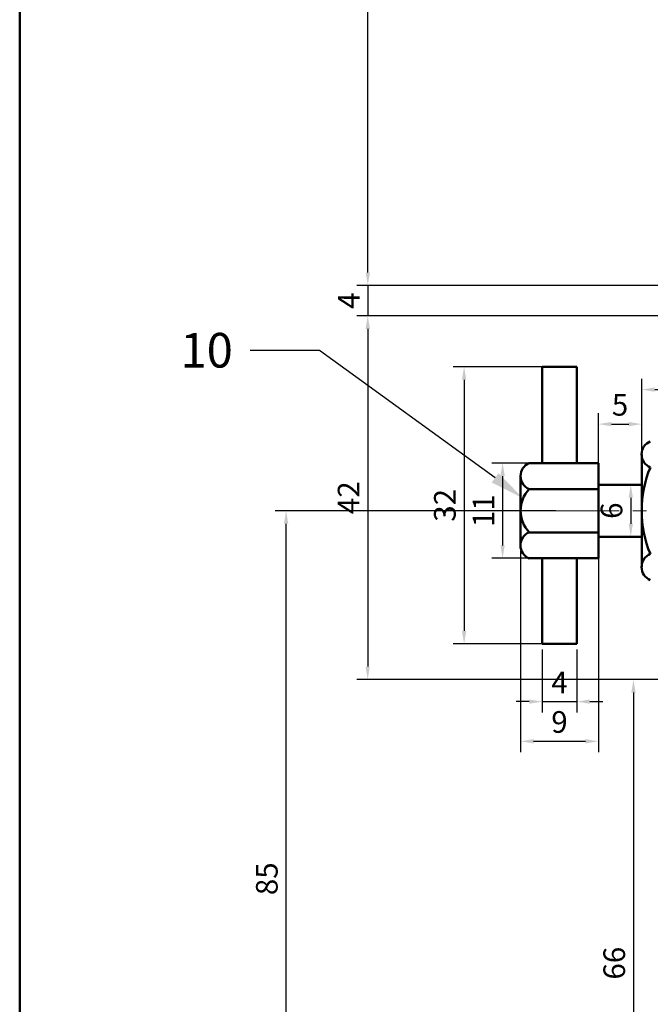
# Model space of a CAD drawing. Units: millimetres. Extents: x -414 to 17, y 81 to 417.
# Tile 2 of 7: x -414 to -341, y 143 to 257. Entities that reach past the tile are written whole.
import ezdxf
from ezdxf import colors
from ezdxf.entities.mleader import LeaderData, LeaderLine
from ezdxf.math import Vec2, Vec3

# ---------------------------------------------------------------- set-up
doc = ezdxf.new("R2010")
doc.units = ezdxf.units.MM
doc.header["$LTSCALE"] = 0.5
doc.linetypes.add('CENTER', pattern=[50.8, 31.75, -6.35, 6.35, -6.35])
for name, color, linetype, lineweight in [('M-CNTR', 1, 'CENTER', 18), ('M-DIMS', 2, 'Continuous', 25), ('M-OUTL', 7, 'Continuous', 50)]:
    doc.layers.add(name, color=color, linetype=linetype, lineweight=lineweight)
doc.styles.get("Standard").update_dxf_attribs({"font": 'arial.ttf'})
doc.dimstyles.new('ISO-25', dxfattribs={"dimtxt": 2.5, "dimasz": 1.5, "dimexe": 1.25, "dimexo": 0.625, "dimtad": 1, "dimtoh": 1, "dimdec": 0, "dimtxsty": 'Standard', "dimcen": 2.5, "dimadec": 0, "dimazin": 0, "dimtfac": 1, "dimtdec": 0, "dimtmove": 0, "dimatfit": 3, "dimfxl": 1, "dimarcsym": 0})

# ---------------------------------------------------------------- blocks, each defined once
blk = doc.blocks.new('*D30')
at = {"layer": 'Defpoints', "color": 0, "ltscale": 0.5, "transparency": 16777216}
for p in [(-330.49, 214.44), (-330.49, 209.27), (-342.49, 205.1)]:
    blk.add_point(p, dxfattribs=at)
at = {"layer": 'M-DIMS', "color": 0, "lineweight": -2, "ltscale": 0.5, "transparency": 16777216}
for p, q in [((-342.49, 205.73), (-342.49, 215.69)), ((-330.49, 209.89), (-330.49, 215.69)), ((-340.99, 214.44), (-331.99, 214.44))]:
    blk.add_line(p, q, dxfattribs=at)
at = {"layer": 'M-DIMS', "color": 0, "ltscale": 0.5, "transparency": 16777216}
for points in [[(-340.99, 214.69), (-340.99, 214.19), (-342.49, 214.44)], [(-331.99, 214.69), (-331.99, 214.19), (-330.49, 214.44)]]:
    blk.add_solid(points, dxfattribs=at)
at = {"layer": 'M-DIMS', "color": 0, "ltscale": 0.5, "transparency": 16777216, "insert": (-336.49, 216.32), "char_height": 2.5, "attachment_point": 5}
blk.add_mtext('12', dxfattribs=at)
blk = doc.blocks.new('*D32')
at = {"layer": 'Defpoints', "color": 0, "ltscale": 0.5, "transparency": 16777216}
for p in [(-344.99, 203.46), (-344.99, 197.46), (-343.75, 197.46)]:
    blk.add_point(p, dxfattribs=at)
at = {"layer": 'M-DIMS', "color": 0, "lineweight": -2, "ltscale": 0.5, "transparency": 16777216}
for p, q in [((-344.37, 203.46), (-342.5, 203.46)), ((-343.75, 201.96), (-343.75, 198.96)), ((-344.37, 197.46), (-342.5, 197.46))]:
    blk.add_line(p, q, dxfattribs=at)
at = {"layer": 'M-DIMS', "color": 0, "ltscale": 0.5, "transparency": 16777216}
for points in [[(-344, 201.96), (-343.5, 201.96), (-343.75, 203.46)], [(-344, 198.96), (-343.5, 198.96), (-343.75, 197.46)]]:
    blk.add_solid(points, dxfattribs=at)
at = {"layer": 'M-DIMS', "color": 0, "ltscale": 0.5, "transparency": 16777216, "insert": (-345.65, 200.46), "char_height": 2.5, "attachment_point": 5, "rotation": 90}
blk.add_mtext('6', dxfattribs=at)
blk = doc.blocks.new('*D33')
at = {"layer": 'Defpoints', "color": 0, "ltscale": 0.5, "transparency": 16777216}
for p in [(-342.49, 210.46), (-347.49, 203.46), (-342.49, 203.46)]:
    blk.add_point(p, dxfattribs=at)
at = {"layer": 'M-DIMS', "color": 0, "lineweight": -2, "ltscale": 0.5, "transparency": 16777216}
for p, q in [((-347.49, 204.09), (-347.49, 211.71)), ((-342.49, 204.09), (-342.49, 211.71)), ((-345.99, 210.46), (-343.99, 210.46))]:
    blk.add_line(p, q, dxfattribs=at)
at = {"layer": 'M-DIMS', "color": 0, "ltscale": 0.5, "transparency": 16777216}
for points in [[(-345.99, 210.71), (-345.99, 210.21), (-347.49, 210.46)], [(-343.99, 210.71), (-343.99, 210.21), (-342.49, 210.46)]]:
    blk.add_solid(points, dxfattribs=at)
at = {"layer": 'M-DIMS', "color": 0, "ltscale": 0.5, "transparency": 16777216, "insert": (-344.99, 212.36), "char_height": 2.5, "attachment_point": 5}
blk.add_mtext('5', dxfattribs=at)
blk = doc.blocks.new('*D34')
at = {"layer": 'Defpoints', "color": 0, "ltscale": 0.5, "transparency": 16777216}
for p in [(-353.99, 185.08), (-349.99, 185.08), (-349.99, 178.41)]:
    blk.add_point(p, dxfattribs=at)
at = {"layer": 'M-DIMS', "color": 0, "lineweight": -2, "ltscale": 0.5, "transparency": 16777216}
for p, q in [((-353.99, 184.45), (-353.99, 177.16)), ((-349.99, 184.45), (-349.99, 177.16)), ((-355.49, 178.41), (-356.99, 178.41)), ((-353.99, 178.41), (-349.99, 178.41)), ((-348.49, 178.41), (-346.99, 178.41))]:
    blk.add_line(p, q, dxfattribs=at)
at = {"layer": 'M-DIMS', "color": 0, "ltscale": 0.5, "transparency": 16777216}
for points in [[(-355.49, 178.66), (-355.49, 178.16), (-353.99, 178.41)], [(-348.49, 178.66), (-348.49, 178.16), (-349.99, 178.41)]]:
    blk.add_solid(points, dxfattribs=at)
at = {"layer": 'M-DIMS', "color": 0, "ltscale": 0.5, "transparency": 16777216, "insert": (-351.99, 180.29), "char_height": 2.5, "attachment_point": 5}
blk.add_mtext('4', dxfattribs=at)
blk = doc.blocks.new('*D35')
at = {"layer": 'Defpoints', "color": 0, "ltscale": 0.5, "transparency": 16777216}
for p in [(-356.49, 196.46), (-347.49, 196.46), (-347.49, 173.83)]:
    blk.add_point(p, dxfattribs=at)
at = {"layer": 'M-DIMS', "color": 0, "lineweight": -2, "ltscale": 0.5, "transparency": 16777216}
for p, q in [((-356.49, 195.84), (-356.49, 172.58)), ((-347.49, 195.84), (-347.49, 172.58)), ((-354.99, 173.83), (-348.99, 173.83))]:
    blk.add_line(p, q, dxfattribs=at)
at = {"layer": 'M-DIMS', "color": 0, "ltscale": 0.5, "transparency": 16777216}
for points in [[(-354.99, 174.08), (-354.99, 173.58), (-356.49, 173.83)], [(-348.99, 174.08), (-348.99, 173.58), (-347.49, 173.83)]]:
    blk.add_solid(points, dxfattribs=at)
at = {"layer": 'M-DIMS', "color": 0, "ltscale": 0.5, "transparency": 16777216, "insert": (-351.99, 175.74), "char_height": 2.5, "attachment_point": 5}
blk.add_mtext('9', dxfattribs=at)
blk = doc.blocks.new('*D36')
at = {"layer": 'Defpoints', "color": 0, "ltscale": 0.5, "transparency": 16777216}
for p in [(-351.99, 217.08), (-363.01, 185.08), (-351.99, 185.08)]:
    blk.add_point(p, dxfattribs=at)
at = {"layer": 'M-DIMS', "color": 0, "lineweight": -2, "ltscale": 0.5, "transparency": 16777216}
for p, q in [((-352.62, 217.08), (-364.26, 217.08)), ((-363.01, 215.58), (-363.01, 186.58)), ((-352.62, 185.08), (-364.26, 185.08))]:
    blk.add_line(p, q, dxfattribs=at)
at = {"layer": 'M-DIMS', "color": 0, "ltscale": 0.5, "transparency": 16777216}
for points in [[(-363.26, 215.58), (-362.76, 215.58), (-363.01, 217.08)], [(-363.26, 186.58), (-362.76, 186.58), (-363.01, 185.08)]]:
    blk.add_solid(points, dxfattribs=at)
at = {"layer": 'M-DIMS', "color": 0, "ltscale": 0.5, "transparency": 16777216, "insert": (-364.91, 201.08), "char_height": 2.5, "attachment_point": 5, "rotation": 90}
blk.add_mtext('32', dxfattribs=at)
blk = doc.blocks.new('*D37')
at = {"layer": 'Defpoints', "color": 0, "ltscale": 0.5, "transparency": 16777216}
for p in [(-338.49, 222.96), (-374.15, 180.96), (-308.49, 180.96)]:
    blk.add_point(p, dxfattribs=at)
at = {"layer": 'M-DIMS', "color": 0, "lineweight": -2, "ltscale": 0.5, "transparency": 16777216}
for p, q in [((-339.12, 222.96), (-375.4, 222.96)), ((-374.15, 221.46), (-374.15, 182.46)), ((-309.12, 180.96), (-375.4, 180.96))]:
    blk.add_line(p, q, dxfattribs=at)
at = {"layer": 'M-DIMS', "color": 0, "ltscale": 0.5, "transparency": 16777216}
for points in [[(-374.4, 221.46), (-373.9, 221.46), (-374.15, 222.96)], [(-374.4, 182.46), (-373.9, 182.46), (-374.15, 180.96)]]:
    blk.add_solid(points, dxfattribs=at)
at = {"layer": 'M-DIMS', "color": 0, "ltscale": 0.5, "transparency": 16777216, "insert": (-376.03, 201.96), "char_height": 2.5, "attachment_point": 5, "rotation": 90}
blk.add_mtext('42', dxfattribs=at)
blk = doc.blocks.new('*D38')
at = {"layer": 'Defpoints', "color": 0, "ltscale": 0.5, "transparency": 16777216}
for p in [(-333.78, 226.46), (-374.14, 222.96), (-333.78, 222.96)]:
    blk.add_point(p, dxfattribs=at)
at = {"layer": 'M-DIMS', "color": 0, "lineweight": -2, "ltscale": 0.5, "transparency": 16777216}
for p, q in [((-374.14, 227.96), (-374.14, 229.46)), ((-334.4, 226.46), (-375.39, 226.46)), ((-374.14, 226.46), (-374.14, 222.96)), ((-334.4, 222.96), (-375.39, 222.96)), ((-374.14, 221.46), (-374.14, 219.96))]:
    blk.add_line(p, q, dxfattribs=at)
at = {"layer": 'M-DIMS', "color": 0, "ltscale": 0.5, "transparency": 16777216}
for points in [[(-374.39, 227.96), (-373.89, 227.96), (-374.14, 226.46)], [(-374.39, 221.46), (-373.89, 221.46), (-374.14, 222.96)]]:
    blk.add_solid(points, dxfattribs=at)
at = {"layer": 'M-DIMS', "color": 0, "ltscale": 0.5, "transparency": 16777216, "insert": (-376.02, 224.71), "char_height": 2.5, "attachment_point": 5, "rotation": 90}
blk.add_mtext('4', dxfattribs=at)
blk = doc.blocks.new('*D39')
at = {"layer": 'Defpoints', "color": 0, "ltscale": 0.5, "transparency": 16777216}
for p in [(-374.14, 356.47), (-308.49, 356.47), (-361.11, 226.46)]:
    blk.add_point(p, dxfattribs=at)
at = {"layer": 'M-DIMS', "color": 0, "lineweight": -2, "ltscale": 0.5, "transparency": 16777216}
for p, q in [((-309.12, 356.47), (-375.39, 356.47)), ((-374.14, 227.96), (-374.14, 354.97)), ((-361.74, 226.46), (-375.39, 226.46))]:
    blk.add_line(p, q, dxfattribs=at)
at = {"layer": 'M-DIMS', "color": 0, "ltscale": 0.5, "transparency": 16777216}
for points in [[(-374.39, 354.97), (-373.89, 354.97), (-374.14, 356.47)], [(-374.39, 227.96), (-373.89, 227.96), (-374.14, 226.46)]]:
    blk.add_solid(points, dxfattribs=at)
at = {"layer": 'M-DIMS', "color": 0, "ltscale": 0.5, "transparency": 16777216, "insert": (-376.05, 291.46), "char_height": 2.5, "attachment_point": 5, "rotation": 90}
blk.add_mtext('130', dxfattribs=at)
blk = doc.blocks.new('*D40')
at = {"layer": 'Defpoints', "color": 0, "ltscale": 0.5, "transparency": 16777216}
for p in [(-351.49, 205.96), (-358.56, 194.96), (-351.49, 194.96)]:
    blk.add_point(p, dxfattribs=at)
at = {"layer": 'M-DIMS', "color": 0, "lineweight": -2, "ltscale": 0.5, "transparency": 16777216}
for p, q in [((-352.12, 205.96), (-359.81, 205.96)), ((-358.56, 204.46), (-358.56, 196.46)), ((-352.12, 194.96), (-359.81, 194.96))]:
    blk.add_line(p, q, dxfattribs=at)
at = {"layer": 'M-DIMS', "color": 0, "ltscale": 0.5, "transparency": 16777216}
for points in [[(-358.81, 204.46), (-358.31, 204.46), (-358.56, 205.96)], [(-358.81, 196.46), (-358.31, 196.46), (-358.56, 194.96)]]:
    blk.add_solid(points, dxfattribs=at)
at = {"layer": 'M-DIMS', "color": 0, "ltscale": 0.5, "transparency": 16777216, "insert": (-360.44, 200.46), "char_height": 2.5, "attachment_point": 5, "rotation": 90}
blk.add_mtext('11', dxfattribs=at)
blk = doc.blocks.new('*D41')
at = {"layer": 'Defpoints', "color": 0, "ltscale": 0.5, "transparency": 16777216}
for p in [(-383.58, 200.46), (-351.8, 200.46), (-308.49, 115.46)]:
    blk.add_point(p, dxfattribs=at)
at = {"layer": 'M-DIMS', "color": 0, "lineweight": -2, "ltscale": 0.5, "transparency": 16777216}
for p, q in [((-352.42, 200.46), (-384.83, 200.46)), ((-383.58, 116.96), (-383.58, 198.96)), ((-309.12, 115.46), (-384.83, 115.46))]:
    blk.add_line(p, q, dxfattribs=at)
at = {"layer": 'M-DIMS', "color": 0, "ltscale": 0.5, "transparency": 16777216}
for points in [[(-383.83, 198.96), (-383.33, 198.96), (-383.58, 200.46)], [(-383.83, 116.96), (-383.33, 116.96), (-383.58, 115.46)]]:
    blk.add_solid(points, dxfattribs=at)
at = {"layer": 'M-DIMS', "color": 0, "ltscale": 0.5, "transparency": 16777216, "insert": (-385.48, 157.96), "char_height": 2.5, "attachment_point": 5, "rotation": 90}
blk.add_mtext('85', dxfattribs=at)
blk = doc.blocks.new('*D45')
at = {"layer": 'Defpoints', "color": 0, "ltscale": 0.5, "transparency": 16777216}
for p in [(-342.26, 180.96), (-343.44, 115.46), (-342.26, 115.46)]:
    blk.add_point(p, dxfattribs=at)
at = {"layer": 'M-DIMS', "color": 0, "lineweight": -2, "ltscale": 0.5, "transparency": 16777216}
for p, q in [((-342.88, 180.96), (-344.69, 180.96)), ((-343.44, 179.46), (-343.44, 116.96)), ((-342.88, 115.46), (-344.69, 115.46))]:
    blk.add_line(p, q, dxfattribs=at)
at = {"layer": 'M-DIMS', "color": 0, "ltscale": 0.5, "transparency": 16777216}
for points in [[(-343.69, 179.46), (-343.19, 179.46), (-343.44, 180.96)], [(-343.69, 116.96), (-343.19, 116.96), (-343.44, 115.46)]]:
    blk.add_solid(points, dxfattribs=at)
at = {"layer": 'M-DIMS', "color": 0, "ltscale": 0.5, "transparency": 16777216, "insert": (-345.34, 148.21), "char_height": 2.5, "attachment_point": 5, "rotation": 90}
blk.add_mtext('66', dxfattribs=at)

msp = doc.modelspace()

# ---------------------------------------------------------------- linework, layer by layer
at = {"layer": 'M-CNTR', "ltscale": 0.5}
msp.add_line((-365.73, 200.46), (-283.99, 200.46), dxfattribs=at)
at = {"layer": 'M-OUTL', "ltscale": 0.5}
for p, q in [((-353.99, 217.08), (-353.99, 205.96)), ((-353.99, 217.08), (-349.99, 217.08)), ((-349.99, 217.08), (-349.99, 205.96)), ((-342.49, 193.96), (-342.49, 206.96)), ((-355.49, 205.96), (-347.49, 205.96)), ((-347.49, 194.96), (-347.49, 205.96)), ((-356.49, 196.46), (-356.49, 204.46)), ((-355.49, 202.96), (-347.49, 202.96)), ((-347.49, 197.46), (-347.49, 203.46)), ((-347.49, 203.46), (-342.49, 203.46)), ((-342.49, 197.46), (-342.49, 203.46)), ((-342.49, 197.96), (-342.49, 202.96)), ((-355.49, 197.96), (-347.49, 197.96)), ((-347.49, 197.46), (-342.49, 197.46)), ((-355.49, 194.96), (-347.49, 194.96)), ((-353.99, 194.96), (-353.99, 185.08)), ((-349.99, 194.96), (-349.99, 185.08)), ((-353.99, 185.08), (-349.99, 185.08))]:
    msp.add_line(p, q, dxfattribs=at)
msp.add_lwpolyline([(-414.36, 417.09), (16.87, 417.09), (16.87, 80.66), (-414.36, 80.66)], close=True, dxfattribs=at)
for centre, radius, start, end in [((-340.87, 206.96), 1.63, 112.6199, 247.3801), ((-354.87, 204.46), 1.62, 112.6199, 247.3801), ((-329.49, 200.46), 13, 157.3801, 202.6199), ((-352.87, 200.46), 3.62, 136.3972, 223.6028), ((-354.87, 196.46), 1.63, 112.6199, 247.3801), ((-340.87, 193.96), 1.63, 112.6199, 247.3801)]:
    msp.add_arc(centre, radius, start, end, dxfattribs=at)

# ---------------------------------------------------------------- dimensions: what is measured, and where the dimension line sits
at = {"layer": 'M-DIMS', "ltscale": 0.5}
for base, p1, p2, picture, middle in [((-374.14, 356.47), (-361.11, 226.46), (-308.49, 356.47), '*D39', (-376.05, 291.46)), ((-374.14409387, 222.96126483), (-333.77523436, 226.46126483), (-333.77523436, 222.96126483), '*D38', (-376.01909387, 224.71126483)), ((-374.15, 180.96), (-338.49, 222.96), (-308.49, 180.96), '*D37', (-376.03, 201.96)), ((-363.01, 185.08), (-351.99, 217.08), (-351.99, 185.08), '*D36', (-364.91, 201.08)), ((-358.56, 194.96), (-351.49, 205.96), (-351.49, 194.96), '*D40', (-360.44, 200.46)), ((-343.75, 197.46), (-344.99, 203.46), (-344.99, 197.46), '*D32', (-345.65, 200.46)), ((-383.58, 200.46), (-308.49, 115.46), (-351.8, 200.46), '*D41', (-385.48, 157.96)), ((-343.43816969, 115.46126483), (-342.25706478, 180.96126483), (-342.25706478, 115.46126483), '*D45', (-345.33960216, 148.21126483))]:
    dim = msp.add_linear_dim(base=base, p1=p1, p2=p2, angle=90, dimstyle='ISO-25', override={"dimclrd": 0, "dimclre": 0, "dimclrt": 0}, dxfattribs=at)
    dim.commit()
    dim.dimension.update_dxf_attribs({"geometry": picture, "text_midpoint": middle})
for base, p1, p2, picture, middle in [((-330.49, 214.44), (-342.49, 205.1), (-330.49, 209.27), '*D30', (-336.49, 216.32)), ((-342.49, 210.46), (-347.49, 203.46), (-342.49, 203.46), '*D33', (-344.99, 212.36))]:
    dim = msp.add_linear_dim(base=base, p1=p1, p2=p2, dimstyle='ISO-25', override={"dimclrd": 0, "dimclre": 0, "dimclrt": 0}, dxfattribs=at)
    dim.commit()
    dim.dimension.update_dxf_attribs({"geometry": picture, "text_midpoint": middle})
for base, p1, p2, picture, middle in [((-347.49, 173.83), (-356.49, 196.46), (-347.49, 196.46), '*D35', (-351.99, 173.83)), ((-349.99, 178.41), (-353.99, 185.08), (-349.99, 185.08), '*D34', (-351.99, 178.41))]:
    dim = msp.add_linear_dim(base=base, p1=p1, p2=p2, dimstyle='ISO-25', override={"dimclrd": 0, "dimclre": 0, "dimclrt": 0}, dxfattribs=at)
    dim.commit()
    dim.dimension.update_dxf_attribs({"geometry": picture, "text_midpoint": middle, "dimtype": 160})

# ---------------------------------------------------------------- leaders
ml = msp.add_multileader_mtext('Standard', dxfattribs=at)
ml.set_content('10', color=256)
ml.set_leader_properties()
ml.build(insert=Vec2(0, 0))
ctx = ml.context
ctx.base_point, ctx.plane_origin = Vec3(-397.07, 218.96), Vec3(-356.19, 201.9)
ctx.text_align_type = 2
notes = []
notes.append((ctx, [(0, (1, 1, 0), (-379.73, 218.96), (-1, 0), 8, [(0, [(-356.19, 201.9)], 0, [])])]))
ctx.mtext.insert, ctx.mtext.alignment, ctx.mtext.flow_direction = Vec3(-389.73, 220.99), 3, 5
for ctx, leaders in notes:
    for number, flags, end, landing, length, lines in leaders:
        leader = LeaderData()
        leader.index, (leader.has_last_leader_line, leader.has_dogleg_vector, leader.attachment_direction) = number, flags
        leader.last_leader_point, leader.dogleg_vector, leader.dogleg_length = Vec3(end), Vec3(landing), length
        for number, points, colour, breaks in lines:
            line = LeaderLine()
            line.index, line.vertices, line.color, line.breaks = number, Vec3.list(points), colors.encode_raw_color(colour), breaks
            leader.lines.append(line)
        ctx.leaders.append(leader)

doc.saveas('drawing.dxf')
